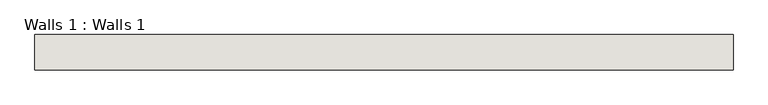
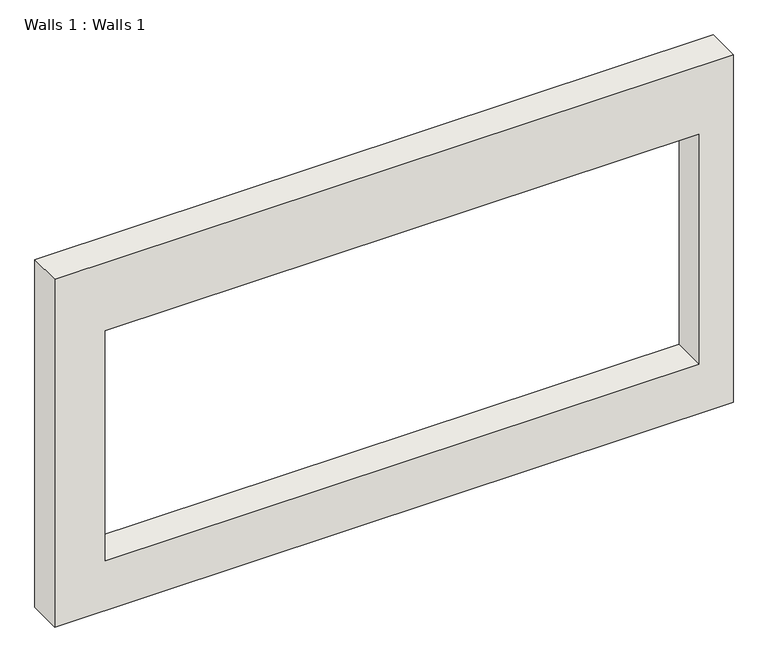
"""IFC4 building model written with IfcOpenShell, lengths in millimetres: wall geometry, Walls 1 : Walls 1."""

from ifc_helpers import new_model, si_unit, frame, origin, place, context, project, spatial, polyline, outline, extrude, source, transform, mapped, element, save


def walls_1_walls_1_1a52f32e(model_context):
    return source(origin(), model_context, "Body", "SweptSolid", [
        extrude(outline(polyline([(7849.0933487, -197.9561565), (7849.0933487, -6243.1561565), (4572.0, -6243.1561565), (4572.0, -197.9561565), (7849.0933487, -197.9561565)]), holes=[polyline([(7206.3339439, -5792.4012139), (7206.3339439, -502.7561565), (5040.3392215, -502.7561565), (5040.3392215, -5792.4012139), (7206.3339439, -5792.4012139)])]), frame((0.0, 1141.3485991, 0.0), z_axis=(0.0, 1.0, 0.0), x_axis=(0.0, 0.0, 1.0)), (0.0, 0.0, 1.0), 304.8),
    ])


if __name__ == "__main__":
    model = new_model("IFC4")
    model_context = context("Model", 3, world=origin())
    ifc_project = project(units=[si_unit("LENGTHUNIT", "METRE", prefix="MILLI")], contexts=[model_context])
    site = spatial("IfcSite", under=ifc_project)
    building = spatial("IfcBuilding", under=site)
    placement = place(None, origin())
    walls_1_walls_1_shape = walls_1_walls_1_1a52f32e(model_context)
    element("IfcWall", 1, ObjectType="Walls 1 : Walls 1", at=placement, inside=building, context=model_context, shape_type="MappedRepresentation", body=[
        mapped(walls_1_walls_1_shape, transform((0.0, 0.0, 0.0), x_axis=(1.0, 0.0, 0.0), y_axis=(0.0, 1.0, 0.0), z_axis=(0.0, 0.0, 1.0))),
    ])
    save(model, "model.ifc")

# Revit data of these elements
# Element 1 (IfcWall, "Walls 1 : Walls 1")
#   Materials on its faces: "Default Wall"
# Materials
#   "Default Wall": colour RGB 128 128 128, transparency 0
